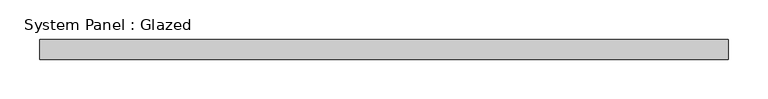
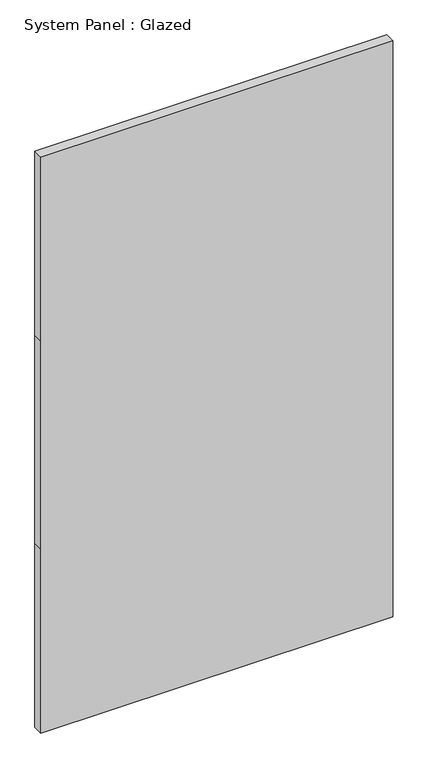
"""IFC4 building model written with IfcOpenShell, lengths in millimetres: plate geometry, System Panel : Glazed."""

from ifc_helpers import new_model, si_unit, frame, origin, place, context, project, spatial, polyline, outline, extrude, source, transform, mapped, element, save


def system_panel_glazed_c3c389f2(model_context):
    return source(origin(), model_context, "Body", "SweptSolid", [
        extrude(outline(polyline([(0.0, -434.975), (0.0, 434.975), (480.6386718, 434.975), (1024.7773437, 434.975), (1505.4160155, 434.975), (1505.4160155, -434.975), (1024.7773437, -434.975), (480.6386718, -434.975), (0.0, -434.975)])), frame((0.0, 19.05, 0.0), z_axis=(0.0, 1.0, 0.0), x_axis=(0.0, 0.0, 1.0)), (0.0, 0.0, 1.0), 25.4),
    ])


if __name__ == "__main__":
    model = new_model("IFC4")
    model_context = context("Model", 3, world=origin())
    ifc_project = project(units=[si_unit("LENGTHUNIT", "METRE", prefix="MILLI")], contexts=[model_context])
    site = spatial("IfcSite", under=ifc_project)
    building = spatial("IfcBuilding", under=site)
    placement = place(None, origin())
    system_panel_glazed_shape = system_panel_glazed_c3c389f2(model_context)
    element("IfcPlate", 1, ObjectType="System Panel : Glazed", at=placement, inside=building, context=model_context, shape_type="MappedRepresentation", body=[
        mapped(system_panel_glazed_shape, transform((0.0, 0.0, 0.0), x_axis=(1.0, 0.0, 0.0), y_axis=(0.0, 1.0, 0.0), z_axis=(0.0, 0.0, 1.0))),
    ])
    save(model, "model.ifc")

# Revit data of these elements
# Type "System Panel : Glazed"
#   Construction Type Id = "GSP4R"
#   Analytic Construction = "1/8 in Pilkington single glazing"
#   Visual Light Transmittance = 0.9
#   Solar Heat Gain Coefficient = 0.86
#   Heat Transfer Coefficient (U) = 1.18115 BTU/(h·ft²·°F)
#   Define Thermal Properties by = 1
# Element 1 (IfcPlate, "System Panel : Glazed")
#   Materials on its faces: "Glass"
# Materials
#   "Glass": class "Glass", colour RGB 0 128 192, transparency 0.75, Description = "Soda Lime Glass", Cost = 0
